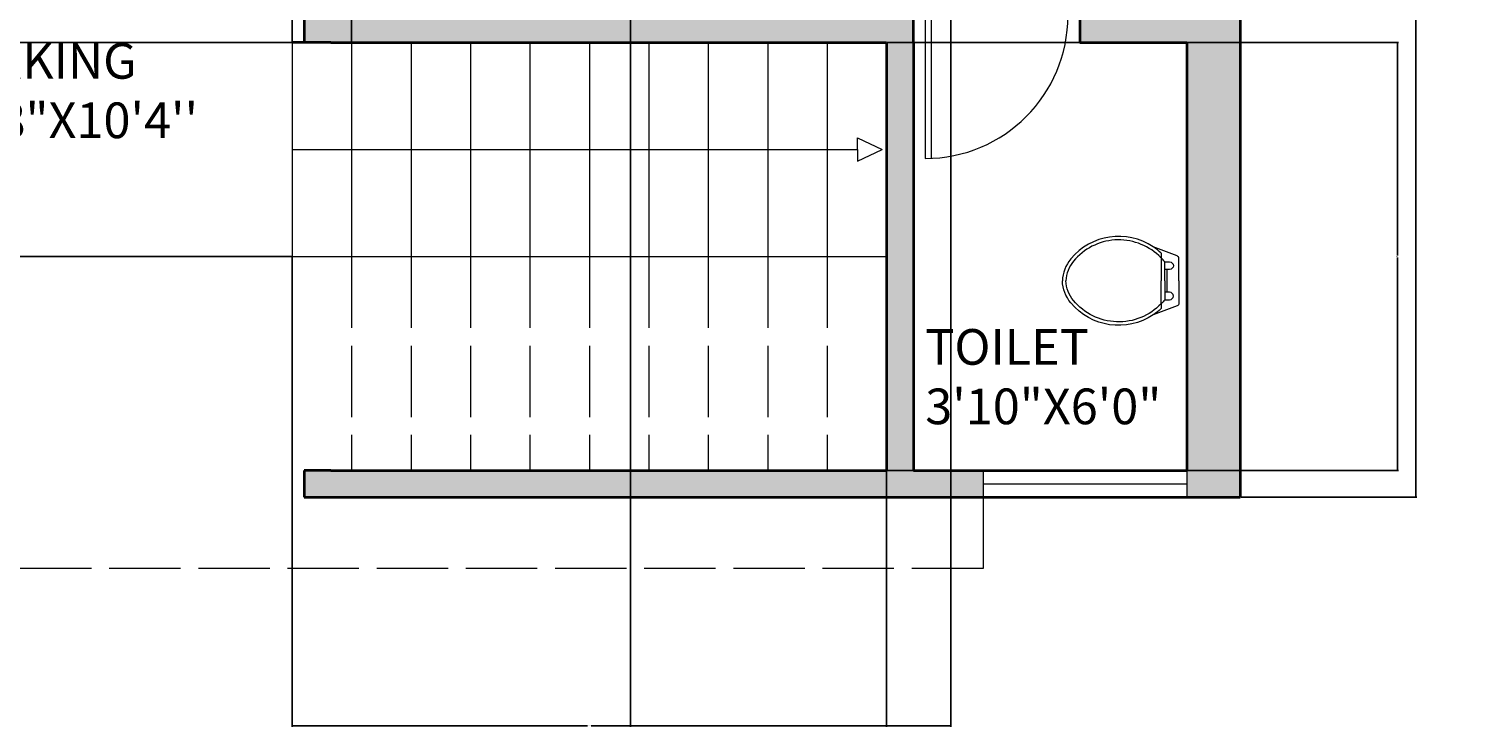
# Model space of a CAD drawing. Units: inches. Extents: x -5 to 366, y -496 to 54.
# Tile 4 of 10: x 121 to 366, y -496 to -378. Entities that reach past the tile are written whole.
import ezdxf

# ---------------------------------------------------------------- set-up
doc = ezdxf.new("R2010")
doc.units = ezdxf.units.IN
doc.header["$MEASUREMENT"] = 0
doc.linetypes.add('ACAD_ISO02W100', pattern=[15, 12, -3])
for name, color, linetype, lineweight in [('A-ANNO-DIMS', 2, 'Continuous', 18), ('A-AREA-IDEN', 7, 'Continuous', 25), ('A-DOOR', 3, 'Continuous', 18), ('A-FLOR-FIXT', 9, 'Continuous', 18), ('A-FLOR-OVHD', 8, 'ACAD_ISO02W100', 18), ('A-FLOR-STRS', 7, 'Continuous', 18), ('A-FLOR-STRS-OVHD', 7, 'ACAD_ISO02W100', 18), ('A-GLAZ', 4, 'Continuous', 18), ('A-WALL', 7, 'Continuous', 35), ('A-WALL-PATT', 252, 'Continuous', 13)]:
    doc.layers.add(name, color=color, linetype=linetype, lineweight=lineweight)
doc.styles.get("Standard").update_dxf_attribs({"font": 'arial.ttf'})
doc.dimstyles.get("Standard").update_dxf_attribs({"dimtxt": 0.18, "dimasz": 0.18, "dimexe": 0.18, "dimexo": 0.0625, "dimgap": 0.09, "dimtad": 0, "dimtih": 1, "dimtoh": 1, "dimdec": 0, "dimzin": 0, "dimdsep": 46, "dimlunit": 3, "dimtxsty": 'Standard', "dimcen": 0.09, "dimadec": 0, "dimazin": 0, "dimtfac": 1, "dimtdec": 0, "dimtofl": 0, "dimtmove": 0, "dimatfit": 3, "dimfxl": 1, "dimtolj": 1, "dimtzin": 0, "dimarcsym": 0})

# ---------------------------------------------------------------- blocks, each defined once
blk = doc.blocks.new('*D3')
at = {"layer": 'A-ANNO-DIMS', "color": 0, "lineweight": -2, "transparency": 16777216}
for p, q in [((325, 26.52), (354.61, 26.52)), ((354.43, 26.34), (354.43, -212.08)), ((354.43, -456.8), (354.43, -218.38)), ((325, -456.98), (354.61, -456.98))]:
    blk.add_line(p, q, dxfattribs=at)
at = {"layer": 'A-ANNO-DIMS', "color": 0, "transparency": 16777216}
for points in [[(354.4, 26.34), (354.46, 26.34), (354.43, 26.52)], [(354.4, -456.8), (354.46, -456.8), (354.43, -456.98)]]:
    blk.add_solid(points, dxfattribs=at)
at = {"layer": 'Defpoints', "color": 0, "transparency": 16777216}
for p in [(324.93, 26.52), (324.93, -456.98), (354.43, -456.98)]:
    blk.add_point(p, dxfattribs=at)
at = {"layer": 'A-ANNO-DIMS', "color": 0, "transparency": 16777216, "insert": (354.43, -215.23), "char_height": 6, "attachment_point": 5}
blk.add_mtext('\\A1;40\'-4"', dxfattribs=at)
blk = doc.blocks.new('DOOR-SWING-24IN')
for p, q in [((-1, 0), (-1, 24)), ((0, 0), (0, 24))]:
    blk.add_line(p, q)
blk.add_arc((0, 0), 24, 90, 180)
blk = doc.blocks.new('WC-PLAN')
for p, q in [((16.62, 12.16), (16.62, 11.34)), ((16.62, 11.34), (16.62, 7.48)), ((16.62, 3.63), (16.62, 7.48)), ((16.62, 3.63), (16.62, 2.81))]:
    blk.add_line(p, q)
for points in [[(15.28, 13.22, 0.383919), (1.41, 11.17, 0.163732), (0, 7.48, 0.359733)], [(16.22, 11.73, 0.431639), (1.86, 10.79, 0.162618), (0.58, 7.48, 0.470877)], [(16.62, 12.16, 0.040937), (15.28, 13.22, 0.163732)], [(19.59, 7.48), (19.59, 11.23, 0.31031), (19.28, 11.68), (15.28, 13.22, 0.209071)], [(16.62, 11.34, 0.014165), (16.22, 11.73, 0.162618)], [(17.22, 10.66, 0.022712), (16.62, 11.34, 0.162618)], [(17.22, 7.48), (17.22, 10.66, 0.022712)], [(17.22, 10.66), (18.04, 10.66, -1), (18.04, 9.41), (17.61, 9.41)], [(15.28, 1.75, -0.383919), (1.41, 3.8, -0.163732), (0, 7.48, -0.359733)], [(16.62, 3.63, -0.448546), (1.86, 4.17, -0.162618), (0.58, 7.48, -0.470877)], [(19.59, 7.48), (19.59, 3.74, -0.31031), (19.28, 3.28), (15.28, 1.75, -0.209071)], [(17.22, 7.48), (17.22, 4.31, -0.476108)], [(17.22, 4.31), (18.04, 4.31, 1), (18.04, 5.56), (17.61, 5.56)], [(16.62, 2.81, -0.040937), (15.28, 1.75, -0.163732)], [(17.22, 4.31, -0.022712), (16.62, 3.63, -0.162618)]]:
    blk.add_lwpolyline(points, format="xyb")
for points in [[(17.61, 9.41), (17.22, 9.41)], [(17.61, 5.56), (17.61, 9.41)], [(17.61, 5.56), (17.22, 5.56)]]:
    blk.add_lwpolyline(points)
blk = doc.blocks.new('*D27')
at = {"layer": 'A-ANNO-DIMS', "color": 0, "lineweight": -2, "transparency": 16777216}
for p, q in [((165.43, -416.54), (165.43, -495.61)), ((265.43, -452.54), (265.43, -495.61)), ((165.61, -495.43), (215.1, -495.43)), ((265.25, -495.43), (215.76, -495.43))]:
    blk.add_line(p, q, dxfattribs=at)
at = {"layer": 'A-ANNO-DIMS', "color": 0, "transparency": 16777216}
for points in [[(165.61, -495.4), (165.61, -495.46), (165.43, -495.43)], [(265.25, -495.4), (265.25, -495.46), (265.43, -495.43)]]:
    blk.add_solid(points, dxfattribs=at)
at = {"layer": 'Defpoints', "color": 0, "transparency": 16777216}
for p in [(165.43, -416.48), (265.43, -452.48), (265.43, -495.43)]:
    blk.add_point(p, dxfattribs=at)
at = {"layer": 'A-ANNO-DIMS', "color": 0, "transparency": 16777216, "insert": (215.43, -495.43), "char_height": 0.18, "attachment_point": 5}
blk.add_mtext('\\A1;8\'-4"', dxfattribs=at)
blk = doc.blocks.new('*D28')
at = {"layer": 'A-ANNO-DIMS', "color": 0, "lineweight": -2, "transparency": 16777216}
for p, q in [((165.37, -380.48), (-4.7, -380.48)), ((-4.52, -380.66), (-4.52, -398.3)), ((-4.52, -416.3), (-4.52, -398.66)), ((165.37, -416.48), (-4.7, -416.48))]:
    blk.add_line(p, q, dxfattribs=at)
at = {"layer": 'A-ANNO-DIMS', "color": 0, "transparency": 16777216}
for points in [[(-4.55, -380.66), (-4.49, -380.66), (-4.52, -380.48)], [(-4.55, -416.3), (-4.49, -416.3), (-4.52, -416.48)]]:
    blk.add_solid(points, dxfattribs=at)
at = {"layer": 'Defpoints', "color": 0, "transparency": 16777216}
for p in [(-4.52, -380.48), (165.43, -380.48), (165.43, -416.48)]:
    blk.add_point(p, dxfattribs=at)
at = {"layer": 'A-ANNO-DIMS', "color": 0, "transparency": 16777216, "insert": (-4.52, -398.48), "char_height": 0.18, "attachment_point": 5}
blk.add_mtext('\\A1;3\'-0"', dxfattribs=at)
blk = doc.blocks.new('*D29')
at = {"layer": 'A-ANNO-DIMS', "color": 0, "lineweight": -2, "transparency": 16777216}
for p, q in [((165.43, -380.42), (165.43, 53.15)), ((165.61, 52.97), (170.03, 52.97)), ((175.25, 52.97), (170.83, 52.97)), ((175.43, -380.42), (175.43, 53.15))]:
    blk.add_line(p, q, dxfattribs=at)
at = {"layer": 'A-ANNO-DIMS', "color": 0, "transparency": 16777216}
for points in [[(165.61, 53), (165.61, 52.94), (165.43, 52.97)], [(175.25, 53), (175.25, 52.94), (175.43, 52.97)]]:
    blk.add_solid(points, dxfattribs=at)
at = {"layer": 'Defpoints', "color": 0, "transparency": 16777216}
for p in [(175.43, 52.97), (165.43, -380.48), (175.43, -380.48)]:
    blk.add_point(p, dxfattribs=at)
at = {"layer": 'A-ANNO-DIMS', "color": 0, "transparency": 16777216, "insert": (170.43, 52.97), "char_height": 0.18, "attachment_point": 5}
blk.add_mtext('\\A1;0\'-10"', dxfattribs=at)
blk = doc.blocks.new('*D30')
at = {"layer": 'A-ANNO-DIMS', "color": 0, "lineweight": -2, "transparency": 16777216}
for p, q in [((265.5, -380.48), (351.56, -380.48)), ((351.38, -380.66), (351.38, -416.3)), ((351.38, -452.3), (351.38, -416.66)), ((265.5, -452.48), (351.56, -452.48))]:
    blk.add_line(p, q, dxfattribs=at)
at = {"layer": 'A-ANNO-DIMS', "color": 0, "transparency": 16777216}
for points in [[(351.35, -380.66), (351.41, -380.66), (351.38, -380.48)], [(351.35, -452.3), (351.41, -452.3), (351.38, -452.48)]]:
    blk.add_solid(points, dxfattribs=at)
at = {"layer": 'Defpoints', "color": 0, "transparency": 16777216}
for p in [(265.43, -380.48), (265.43, -452.48), (351.38, -452.48)]:
    blk.add_point(p, dxfattribs=at)
at = {"layer": 'A-ANNO-DIMS', "color": 0, "transparency": 16777216, "insert": (351.38, -416.48), "char_height": 0.18, "attachment_point": 5}
blk.add_mtext('\\A1;6\'-0"', dxfattribs=at)
blk = doc.blocks.new('*D32')
at = {"layer": 'A-ANNO-DIMS', "color": 0, "lineweight": -2, "transparency": 16777216}
for p, q in [((222.37, -254.15), (222.37, -495.61)), ((276.25, -254.15), (276.25, -495.61)), ((222.55, -495.43), (248.98, -495.43)), ((276.07, -495.43), (249.64, -495.43))]:
    blk.add_line(p, q, dxfattribs=at)
at = {"layer": 'A-ANNO-DIMS', "color": 0, "transparency": 16777216}
for points in [[(222.55, -495.4), (222.55, -495.46), (222.37, -495.43)], [(276.07, -495.4), (276.07, -495.46), (276.25, -495.43)]]:
    blk.add_solid(points, dxfattribs=at)
at = {"layer": 'Defpoints', "color": 0, "transparency": 16777216}
for p in [(222.37, -254.09), (276.25, -254.09), (276.25, -495.43)]:
    blk.add_point(p, dxfattribs=at)
at = {"layer": 'A-ANNO-DIMS', "color": 0, "transparency": 16777216, "insert": (249.31, -495.43), "char_height": 0.18, "attachment_point": 5}
blk.add_mtext('\\A1;4\'-6"', dxfattribs=at)

msp = doc.modelspace()

# ---------------------------------------------------------------- hatches: boundary and pattern name
at = {"layer": 'A-WALL-PATT'}
h = msp.add_hatch(color=256, dxfattribs=at)
h.dxf.hatch_style = 1
h.paths.add_polyline_path([(324.93, 26.52), (21.93, 26.52), (21.93, -456.98), (26.43, -456.98), (26.43, -331.98), (30.93, -331.98), (30.93, -322.98), (30.93, -106.98), (110.93, -106.98), (110.93, -104.73), (110.93, -102.48), (30.93, -102.48), (30.93, 17.52), (138.93, 17.52), (141.18, 17.52), (143.43, 17.52), (183.43, 17.52), (187.93, 17.52), (315.93, 17.52), (315.93, -102.48), (315.93, -106.98), (315.93, -255.48), (171.93, -255.48), (171.93, -155.84), (167.43, -155.84), (167.43, -291.98), (171.93, -291.98), (171.93, -259.98), (315.93, -259.98), (315.93, -375.98), (297.93, -375.98), (297.93, -380.48), (315.93, -380.48), (315.93, -452.48), (315.93, -456.98), (324.93, -456.98)])
h.paths.add_polyline_path([(143.43, -18.48), (143.43, -13.98), (138.93, -13.98), (138.93, -106.98), (187.93, -106.98), (187.93, -102.48), (143.43, -102.48)], flags=17)
h = msp.add_hatch(color=256, dxfattribs=at)
h.dxf.hatch_style = 1
h.paths.add_polyline_path([(187.93, -13.98), (183.43, -13.98), (163.43, -13.98), (163.43, -18.48), (183.43, -18.48), (183.43, -74.48), (185.68, -74.48), (187.93, -74.48)])
h.paths.add_polyline_path([(284.93, -102.48), (215.93, -102.48), (215.93, -104.73), (215.93, -106.98), (280.43, -106.98), (284.93, -106.98)])
h.paths.add_polyline_path([(284.93, -133.23), (280.43, -133.23), (280.43, -154.98), (220.43, -154.98), (220.43, -134.98), (215.93, -134.98), (215.93, -159.48), (284.93, -159.48)])
h.paths.add_polyline_path([(139.43, -322.98), (123.64, -322.98), (123.64, -331.98), (139.43, -331.98)])
h.paths.add_polyline_path([(171.93, -319.98), (167.43, -319.98), (167.43, -331.98), (171.93, -331.98)])
h.paths.add_polyline_path([(269.93, -375.98), (171.93, -375.98), (167.43, -375.98), (167.43, -380.48), (171.93, -380.48), (265.43, -380.48), (265.43, -452.48), (171.93, -452.48), (167.43, -452.48), (167.43, -456.98), (281.67, -456.98), (281.67, -452.48), (269.93, -452.48), (269.93, -380.48)])

# ---------------------------------------------------------------- linework, layer by layer
at = {"layer": 'A-FLOR-OVHD'}
for p, q in [((281.67, -456.98), (281.67, -468.98)), ((281.67, -468.98), (21.93, -468.98))]:
    msp.add_line(p, q, dxfattribs=at)
at = {"layer": 'A-FLOR-STRS'}
for p, q in [((165.43, -380.48), (165.43, -416.48)), ((175.43, -380.48), (175.43, -416.48)), ((185.43, -380.48), (185.43, -416.48)), ((195.43, -380.48), (195.43, -416.48)), ((205.43, -380.48), (205.43, -416.48)), ((215.43, -380.48), (215.43, -416.48)), ((225.43, -380.48), (225.43, -416.48)), ((235.43, -380.48), (235.43, -416.48)), ((245.43, -380.48), (245.43, -416.48)), ((255.43, -380.48), (255.43, -416.48)), ((165.43, -398.48), (260.51, -398.48)), ((260.51, -398.48), (260.51, -396.51)), ((260.51, -396.51), (264.66, -398.48)), ((260.51, -398.48), (260.51, -400.45)), ((260.51, -400.45), (264.66, -398.48)), ((165.43, -416.48), (265.43, -416.48))]:
    msp.add_line(p, q, dxfattribs=at)
at = {"layer": 'A-FLOR-STRS-OVHD'}
for p, q in [((175.43, -416.48), (175.43, -452.48)), ((185.43, -416.48), (185.43, -452.48)), ((195.43, -416.48), (195.43, -452.48)), ((205.43, -416.48), (205.43, -452.48)), ((215.43, -416.48), (215.43, -452.48)), ((225.43, -416.48), (225.43, -452.48)), ((235.43, -416.48), (235.43, -452.48)), ((245.43, -416.48), (245.43, -452.48)), ((255.43, -416.48), (255.43, -452.48))]:
    msp.add_line(p, q, dxfattribs=at)
at = {"layer": 'A-GLAZ'}
for p, q in [((281.67, -452.48), (281.67, -456.98)), ((281.67, -454.73), (315.93, -454.73)), ((315.93, -452.48), (315.93, -456.98))]:
    msp.add_line(p, q, dxfattribs=at)
at = {"layer": 'A-WALL'}
for p, q in [((324.93, 26.52), (324.93, -456.98)), ((167.43, -319.98), (167.43, -380.48)), ((269.93, -380.48), (269.93, -375.98)), ((297.93, -375.98), (297.93, -380.48)), ((171.93, -380.48), (165.43, -380.48)), ((171.93, -380.48), (265.43, -380.48)), ((265.43, -380.48), (265.43, -452.48)), ((269.93, -380.48), (269.93, -452.48)), ((297.93, -380.48), (315.93, -380.48)), ((315.93, -380.48), (315.93, -452.48)), ((167.43, -452.48), (167.43, -456.98)), ((171.93, -452.48), (167.43, -452.48)), ((171.93, -452.48), (265.43, -452.48)), ((269.93, -452.48), (315.93, -452.48)), ((167.43, -456.98), (324.93, -456.98))]:
    msp.add_line(p, q, dxfattribs=at)

# ---------------------------------------------------------------- block references
at = {"layer": 'A-DOOR', "rotation": 180}
msp.add_blockref('DOOR-SWING-24IN', (271.93, -375.98), dxfattribs=at)
at = {"layer": 'A-FLOR-FIXT'}
msp.add_blockref('WC-PLAN', (295, -428.06), dxfattribs=at)

# ---------------------------------------------------------------- texts
at = {"layer": 'A-AREA-IDEN', "char_height": 6, "attachment_point": 1}
for s, insert in [('PARKING\\P11\'8"X10\'4\'\'', (104.68, -380.57)), ('TOILET\\P3\'10"X6\'0"', (271.93, -428.69))]:
    msp.add_mtext(s, dxfattribs=dict(at, insert=insert))

# ---------------------------------------------------------------- dimensions: what is measured, and where the dimension line sits
at = {"layer": 'A-ANNO-DIMS'}
for base, p1, p2, picture, middle in [((175.43, 52.97), (165.43, -380.48), (175.43, -380.48), '*D29', (170.43, 52.97)), ((276.25, -495.43), (222.37, -254.09), (276.25, -254.09), '*D32', (249.31, -495.43)), ((265.43, -495.43), (165.43, -416.48), (265.43, -452.48), '*D27', (215.43, -495.43))]:
    dim = msp.add_linear_dim(base=base, p1=p1, p2=p2, dimstyle='Standard', override={"dimdec": 1, "dimlfac": 1, "dimrnd": 0, "dimzin": 1, "dimdsep": 46, "dimlunit": 4, "dimfrac": 2}, dxfattribs=at)
    dim.commit()
    dim.dimension.update_dxf_attribs({"geometry": picture, "text_midpoint": middle})
for base, p1, p2, override, picture, middle in [((354.42742117, -456.97937362), (324.93325287, 26.52062638), (324.93325287, -456.97937362), {"dimtxt": 6, "dimclrd": 0, "dimclre": 0, "dimclrt": 0}, '*D3', (354.42742117, -215.22937362)), ((-4.52, -380.48), (165.43, -416.48), (165.43, -380.48), {"dimdec": 1, "dimlfac": 1, "dimrnd": 0, "dimzin": 1, "dimdsep": 46, "dimlunit": 4, "dimfrac": 2}, '*D28', (-4.52, -398.48)), ((351.38, -452.48), (265.43, -380.48), (265.43, -452.48), {"dimdec": 1, "dimlfac": 1, "dimrnd": 0, "dimzin": 1, "dimdsep": 46, "dimlunit": 4, "dimfrac": 2}, '*D30', (351.38, -416.48))]:
    dim = msp.add_linear_dim(base=base, p1=p1, p2=p2, angle=90, dimstyle='Standard', override=override, dxfattribs=at)
    dim.commit()
    dim.dimension.update_dxf_attribs({"geometry": picture, "text_midpoint": middle})

doc.saveas('drawing.dxf')
